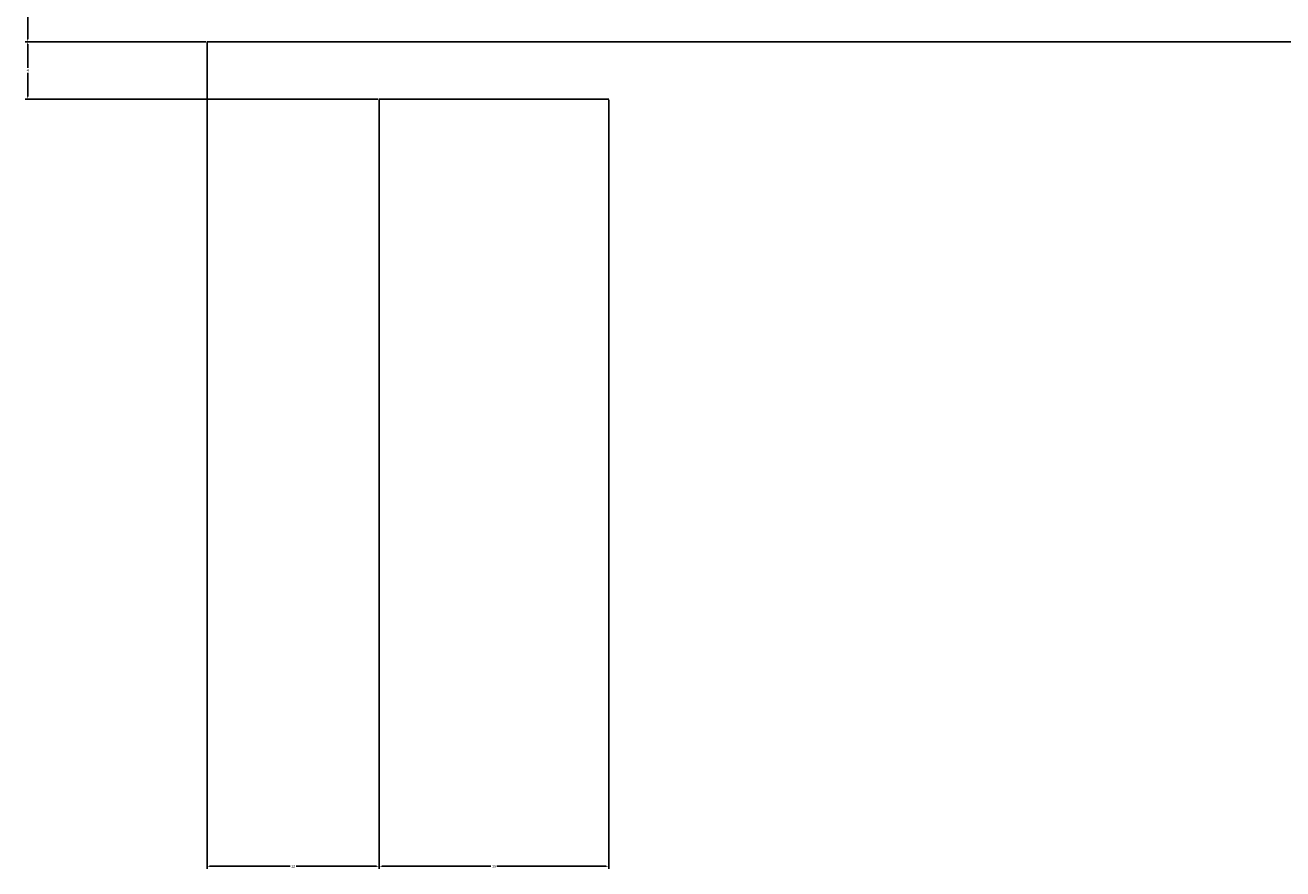
# Model space of a CAD drawing. Units: millimetres. Extents: x 135 to 361, y -58 to 58.
# Tile 1 of 5: x 135 to 223, y -58 to 1. Entities that reach past the tile are written whole.
import ezdxf

# ---------------------------------------------------------------- set-up
doc = ezdxf.new("R2010")
doc.units = ezdxf.units.MM
doc.layers.add('M-CONS', color=8, linetype='Continuous', lineweight=13)
doc.layers.add('M-DIMS', color=2, linetype='Continuous', lineweight=18)
doc.styles.get("Standard").update_dxf_attribs({"font": 'arial.ttf'})
doc.dimstyles.get("Standard").update_dxf_attribs({"dimtxt": 0.18, "dimasz": 0.18, "dimexe": 0.18, "dimexo": 0.0625, "dimgap": 0.09, "dimtad": 0, "dimtih": 1, "dimtoh": 1, "dimdec": 4, "dimzin": 0, "dimdsep": 46, "dimtxsty": 'Standard', "dimcen": 0.09, "dimadec": 0, "dimazin": 0, "dimtfac": 1, "dimtdec": 4, "dimtofl": 0, "dimtmove": 0, "dimatfit": 3, "dimfxl": 1, "dimtolj": 1, "dimtzin": 0, "dimarcsym": 0})

# ---------------------------------------------------------------- blocks, each defined once
blk = doc.blocks.new('*D11')
at = {"layer": 'Defpoints', "color": 0, "transparency": 16777216}
for p in [(135.313, 35), (147.813, 35), (147.813, 0)]:
    blk.add_point(p, dxfattribs=at)
at = {"layer": 'M-DIMS', "color": 0, "lineweight": -2, "transparency": 16777216}
for p, q in [((147.75, 35), (135.133, 35)), ((135.313, 34.82), (135.313, 17.682)), ((135.313, 0.18), (135.313, 17.318)), ((147.75, 0), (135.133, 0))]:
    blk.add_line(p, q, dxfattribs=at)
at = {"layer": 'M-DIMS', "color": 0, "transparency": 16777216}
for points in [[(135.283, 34.82), (135.343, 34.82), (135.313, 35)], [(135.283, 0.18), (135.343, 0.18), (135.313, 0)]]:
    blk.add_solid(points, dxfattribs=at)
at = {"layer": 'M-DIMS', "color": 0, "transparency": 16777216, "insert": (135.313, 17.5), "char_height": 0.18, "attachment_point": 5}
blk.add_mtext('\\A1;35', dxfattribs=at)
blk = doc.blocks.new('*D12')
at = {"layer": 'Defpoints', "color": 0, "transparency": 16777216}
for p in [(159.813, -4), (175.813, -4), (175.813, -57.5)]:
    blk.add_point(p, dxfattribs=at)
at = {"layer": 'M-DIMS', "color": 0, "lineweight": -2, "transparency": 16777216}
for p, q in [((159.813, -4.062), (159.813, -57.68)), ((175.813, -4.062), (175.813, -57.68)), ((159.993, -57.5), (167.602, -57.5)), ((175.633, -57.5), (168.023, -57.5))]:
    blk.add_line(p, q, dxfattribs=at)
at = {"layer": 'M-DIMS', "color": 0, "transparency": 16777216}
for points in [[(159.993, -57.47), (159.993, -57.53), (159.813, -57.5)], [(175.633, -57.47), (175.633, -57.53), (175.813, -57.5)]]:
    blk.add_solid(points, dxfattribs=at)
at = {"layer": 'M-DIMS', "color": 0, "transparency": 16777216, "insert": (167.813, -57.5), "char_height": 0.18, "attachment_point": 5}
blk.add_mtext('\\A1;16', dxfattribs=at)
blk = doc.blocks.new('*D13')
at = {"layer": 'Defpoints', "color": 0, "transparency": 16777216}
for p in [(147.813, 0), (159.813, -4), (159.813, -57.5)]:
    blk.add_point(p, dxfattribs=at)
at = {"layer": 'M-DIMS', "color": 0, "lineweight": -2, "transparency": 16777216}
for p, q in [((147.813, -0.062), (147.813, -57.68)), ((159.813, -4.062), (159.813, -57.68)), ((147.993, -57.5), (153.603, -57.5)), ((159.633, -57.5), (154.022, -57.5))]:
    blk.add_line(p, q, dxfattribs=at)
at = {"layer": 'M-DIMS', "color": 0, "transparency": 16777216}
for points in [[(147.993, -57.47), (147.993, -57.53), (147.813, -57.5)], [(159.633, -57.47), (159.633, -57.53), (159.813, -57.5)]]:
    blk.add_solid(points, dxfattribs=at)
at = {"layer": 'M-DIMS', "color": 0, "transparency": 16777216, "insert": (153.813, -57.5), "char_height": 0.18, "attachment_point": 5}
blk.add_mtext('\\A1;12', dxfattribs=at)
blk = doc.blocks.new('*D14')
at = {"layer": 'Defpoints', "color": 0, "transparency": 16777216}
for p in [(147.812543, 0), (135.312543, -4), (159.812543, -4)]:
    blk.add_point(p, dxfattribs=at)
at = {"layer": 'M-DIMS', "color": 0, "lineweight": -2, "transparency": 16777216}
for p, q in [((147.750043, 0), (135.132543, 0)), ((135.312543, -0.18), (135.312543, -1.82)), ((135.312543, -3.82), (135.312543, -2.18)), ((159.750043, -4), (135.132543, -4))]:
    blk.add_line(p, q, dxfattribs=at)
at = {"layer": 'M-DIMS', "color": 0, "transparency": 16777216}
for points in [[(135.282543, -0.18), (135.342543, -0.18), (135.312543, 0)], [(135.282543, -3.82), (135.342543, -3.82), (135.312543, -4)]]:
    blk.add_solid(points, dxfattribs=at)
at = {"layer": 'M-DIMS', "color": 0, "transparency": 16777216, "insert": (135.312543, -2), "char_height": 0.18, "attachment_point": 5}
blk.add_mtext('\\A1;4', dxfattribs=at)

msp = doc.modelspace()

# ---------------------------------------------------------------- linework, layer by layer
at = {"layer": 'M-CONS', "extrusion": (0, -1, 0)}
msp.add_lwpolyline([(167.813, 133.744), (284.813, 145.744), (347.813, 117.744), (347.813, 93.744), (167.813, 93.744)], dxfattribs=at)
for centre, radius in [((167.813, 113.744), 20), ((167.813, 113.744, 4), 8)]:
    msp.add_circle(centre, radius, dxfattribs=at)

# ---------------------------------------------------------------- dimensions: what is measured, and where the dimension line sits
at = {"layer": 'M-DIMS'}
for base, p2, picture, middle in [((135.313, 35), (147.813, 35), '*D11', (135.313, 17.5)), ((135.313, -4), (159.813, -4), '*D14', (135.313, -2))]:
    dim = msp.add_linear_dim(base=base, p1=(147.813, 0), p2=p2, angle=90, dimstyle='Standard', override={"dimdec": 0, "dimlfac": 1, "dimrnd": 0, "dimzin": 0, "dimdsep": 46, "dimlunit": 2}, dxfattribs=at)
    dim.commit()
    dim.dimension.update_dxf_attribs({"geometry": picture, "text_midpoint": middle})
for base, p1, p2, picture, middle in [((159.813, -57.5), (147.813, 0), (159.813, -4), '*D13', (153.813, -57.5)), ((175.813, -57.5), (159.813, -4), (175.813, -4), '*D12', (167.813, -57.5))]:
    dim = msp.add_linear_dim(base=base, p1=p1, p2=p2, dimstyle='Standard', override={"dimdec": 0, "dimlfac": 1, "dimrnd": 0, "dimzin": 0, "dimdsep": 46, "dimlunit": 2}, dxfattribs=at)
    dim.commit()
    dim.dimension.update_dxf_attribs({"geometry": picture, "text_midpoint": middle})

doc.saveas('drawing.dxf')
